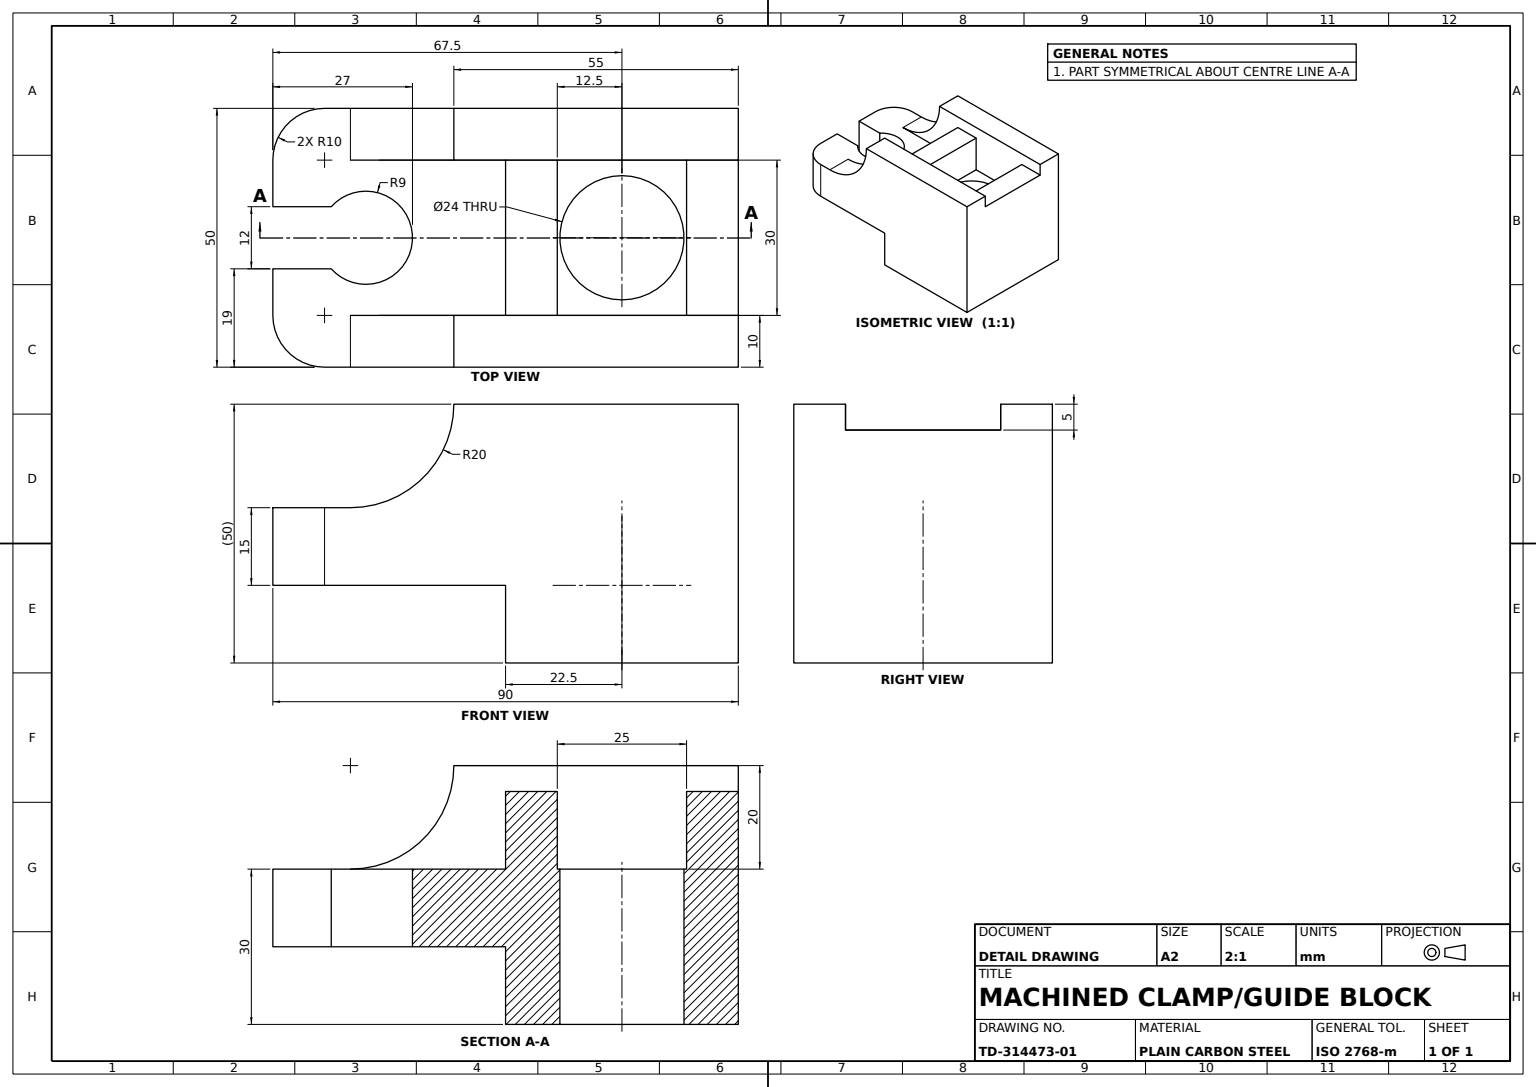
from build123d import *

# Parameters (mm, degrees)
BASE_PLATE_SKETCH_W      = 90
BASE_PLATE_SKETCH_H      = 15
BASE_PLATE_DEPTH         = 50
SIDE_WALL_SKETCH_W       = 45
SIDE_WALL_SKETCH_H       = 15
SIDE_WALL_DEPTH          = 50
RAISED_BLOCK_SKETCH_W    = 55
RAISED_BLOCK_SKETCH_H    = 20
RAISED_BLOCK_DEPTH       = 50
STEP_NOTCH_CUT_DEPTH     = 50
FIRST_ROUNDED_LUG_DEPTH  = 10
SECOND_START             = -10
SECOND_ROUNDED_LUG_DEPTH = 10
SLOT_CUT_DEPTH           = 15
CHANNEL_SKETCH_W         = 30
CHANNEL_SKETCH_H         = 20
CHANNEL_CUT_DEPTH        = 60
RAIL_BOSS_SKETCH_W       = 30
RAIL_BOSS_SKETCH_H       = 20
RAIL_BOSS_DEPTH          = 10
CURVED_RECESS_SKETCH_W   = 10
CURVED_RECESS_SKETCH_H   = 30
CURVED_RECESS_CUT_DEPTH  = 5
BRIDGE_BLOCK_SKETCH_W    = 10
BRIDGE_BLOCK_SKETCH_H    = 30
BRIDGE_BLOCK_DEPTH       = 20
BRIDGE_RELIEF_SKETCH_W   = 10
BRIDGE_RELIEF_SKETCH_H   = 30
BRIDGE_RELIEF_CUT_DEPTH  = 5
BORE_24_SKETCH_R         = 12
BORE_24_DEPTH            = 70


with BuildPart() as part:
    # Base Plate Sketch → Base Plate (new body)
    with BuildSketch(Plane.XY):
        with Locations((45, 7.5)):
            Rectangle(BASE_PLATE_SKETCH_W, BASE_PLATE_SKETCH_H)
    extrude(amount=-BASE_PLATE_DEPTH)

    # Side Wall Sketch → Side Wall (add)
    with BuildSketch(Plane.XY):
        with Locations((67.5, -7.5)):
            Rectangle(SIDE_WALL_SKETCH_W, SIDE_WALL_SKETCH_H)
    extrude(amount=-SIDE_WALL_DEPTH)

    # Raised Block Sketch → Raised Block (add)
    with BuildSketch(Plane.XY):
        with Locations((62.5, 25)):
            Rectangle(RAISED_BLOCK_SKETCH_W, RAISED_BLOCK_SKETCH_H)
    extrude(amount=-RAISED_BLOCK_DEPTH)

    # Step Notch Sketch → Step Notch Cut (cut)
    with BuildSketch(Plane(origin=(0, 15, 0), x_dir=(1, 0, 0), z_dir=(0, 1, 0))):
        with BuildLine():
            Line((10, 50), (0, 50))
            Line((0, 50), (0, 40))
            ThreePointArc((0, 40), (2.928932188, 47.071067812), (10, 50))
        make_face()
        with BuildLine():
            ThreePointArc((10, 0), (2.928932188, 2.928932188), (0, 10))
            Line((0, 10), (0, 0))
            Line((0, 0), (10, 0))
        make_face()
    extrude(amount=-STEP_NOTCH_CUT_DEPTH, mode=Mode.SUBTRACT)

    # First Rounded Lug Sketch → First Rounded Lug (add)
    with BuildSketch(Plane.XY):
        with BuildLine():
            Line((35, 35), (35, 15))
            Line((35, 15), (15, 15))
            ThreePointArc((15, 15), (29.142135624, 20.857864376), (35, 35))
        make_face()
    extrude(amount=-FIRST_ROUNDED_LUG_DEPTH)

    # Second Rounded Lug Sketch → Second Rounded Lug (add)
    with BuildSketch(Plane(origin=(0, 0, -50), x_dir=(-1, 0, 0), z_dir=(0, 0, -1)).offset(SECOND_START)):
        with BuildLine():
            Line((-35, 35), (-35, 15))
            Line((-35, 15), (-15, 15))
            ThreePointArc((-15, 15), (-29.142135624, 20.857864376), (-35, 35))
        make_face()
    extrude(amount=SECOND_ROUNDED_LUG_DEPTH)

    # Slot Sketch → Slot Cut (cut)
    with BuildSketch(Plane(origin=(0, 15, 0), x_dir=(1, 0, 0), z_dir=(0, 1, 0))):
        with BuildLine():
            Line((0, 25), (0, 31))
            Line((0, 31), (11.291796068, 31))
            ThreePointArc((11.291796068, 31), (27, 25), (11.291796068, 19))
            Line((11.291796068, 19), (0, 19))
            Line((0, 19), (0, 25))
        make_face()
    extrude(amount=-SLOT_CUT_DEPTH, mode=Mode.SUBTRACT)

    # Channel Sketch → Channel Cut (cut)
    with BuildSketch(Plane.ZY.offset(-35)):
        with Locations((-25, 25)):
            Rectangle(CHANNEL_SKETCH_W, CHANNEL_SKETCH_H)
    extrude(amount=-CHANNEL_CUT_DEPTH, mode=Mode.SUBTRACT)

    # Rail Boss Sketch → Rail Boss (add)
    with BuildSketch(Plane(origin=(90, 0, 0), x_dir=(0, 0, -1), z_dir=(1, 0, 0))):
        with Locations((25, 25)):
            Rectangle(RAIL_BOSS_SKETCH_W, RAIL_BOSS_SKETCH_H)
    extrude(amount=-RAIL_BOSS_DEPTH)

    # Curved Recess Sketch → Curved Recess Cut (cut)
    with BuildSketch(Plane(origin=(0, 35, 0), x_dir=(1, 0, 0), z_dir=(0, 1, 0))):
        with Locations((85, 25)):
            Rectangle(CURVED_RECESS_SKETCH_W, CURVED_RECESS_SKETCH_H)
    extrude(amount=-CURVED_RECESS_CUT_DEPTH, mode=Mode.SUBTRACT)

    # Bridge Block Sketch → Bridge Block (add)
    with BuildSketch(Plane(origin=(0, 35, 0), x_dir=(1, 0, 0), z_dir=(0, 1, 0))):
        with Locations((50, 25)):
            Rectangle(BRIDGE_BLOCK_SKETCH_W, BRIDGE_BLOCK_SKETCH_H)
    extrude(amount=-BRIDGE_BLOCK_DEPTH)

    # Bridge Relief Sketch → Bridge Relief Cut (cut)
    with BuildSketch(Plane(origin=(0, 35, 0), x_dir=(1, 0, 0), z_dir=(0, 1, 0))):
        with Locations((50, 25)):
            Rectangle(BRIDGE_RELIEF_SKETCH_W, BRIDGE_RELIEF_SKETCH_H)
    extrude(amount=-BRIDGE_RELIEF_CUT_DEPTH, mode=Mode.SUBTRACT)

    # Bore Ø24 Sketch → Bore Ø24 (cut)
    with BuildSketch(Plane(origin=(0, 15, 0), x_dir=(1, 0, 0), z_dir=(0, 1, 0))):
        with Locations(Location((67.5, 25, 0), (0, 0, 270))):
            Circle(BORE_24_SKETCH_R)
    extrude(amount=-BORE_24_DEPTH, mode=Mode.SUBTRACT)


solid = part.part
